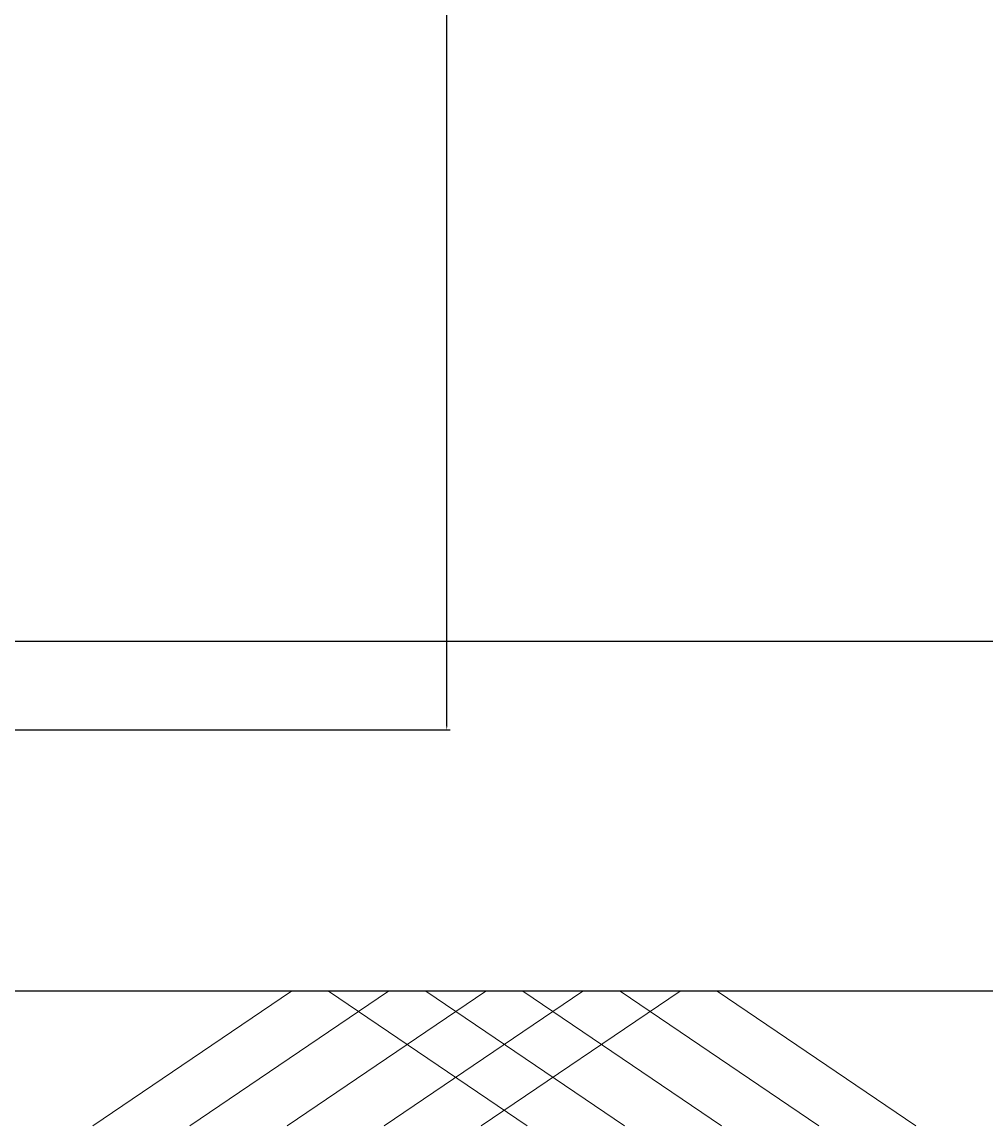
# Model space of a CAD drawing. Units: inches. Extents: x -128 to 854, y -395 to 398.
# Tile 51 of 61: x 368 to 417, y -378 to -322. Entities that reach past the tile are written whole.
import ezdxf

# ---------------------------------------------------------------- set-up
doc = ezdxf.new("R2010")
doc.units = ezdxf.units.IN
doc.header["$MEASUREMENT"] = 0
for name, color, linetype, lineweight in [('A-ANNO-DIMS', 2, 'Continuous', 18), ('C-GRAD', 7, 'Continuous', 25), ('C-GRAD-PATT', 8, 'Continuous', 13)]:
    doc.layers.add(name, color=color, linetype=linetype, lineweight=lineweight)
doc.styles.get("Standard").update_dxf_attribs({"font": 'arial.ttf'})
doc.dimstyles.get("Standard").update_dxf_attribs({"dimtxt": 0.18, "dimasz": 0.18, "dimexe": 0.18, "dimexo": 0.0625, "dimgap": 0.09, "dimtad": 0, "dimtih": 1, "dimtoh": 1, "dimdec": 1, "dimzin": 0, "dimdsep": 46, "dimlunit": 4, "dimtxsty": 'Standard', "dimcen": 0.09, "dimclrd": 1, "dimclre": 2, "dimclrt": 6, "dimadec": 0, "dimazin": 0, "dimtfac": 1, "dimtdec": 1, "dimtofl": 0, "dimtmove": 0, "dimatfit": 3, "dimfxl": 1, "dimtfill": 2, "dimtfillclr": 3, "dimtolj": 1, "dimtzin": 0, "dimarcsym": 0})

# ---------------------------------------------------------------- blocks, each defined once
blk = doc.blocks.new('*D120')
at = {"layer": 'A-ANNO-DIMS', "color": 2, "lineweight": -2, "transparency": 16777216}
for p, q in [((317.902, -178.019), (389.719, -178.019)), ((337.902, -358.019), (389.719, -358.019))]:
    blk.add_line(p, q, dxfattribs=at)
at = {"layer": 'A-ANNO-DIMS', "color": 1, "lineweight": -2, "transparency": 16777216}
for p, q in [((389.539, -178.199), (389.539, -267.837)), ((389.539, -357.839), (389.539, -268.201))]:
    blk.add_line(p, q, dxfattribs=at)
at = {"layer": 'A-ANNO-DIMS', "color": 1, "transparency": 16777216}
for points in [[(389.509, -178.199), (389.569, -178.199), (389.539, -178.019)], [(389.509, -357.839), (389.569, -357.839), (389.539, -358.019)]]:
    blk.add_solid(points, dxfattribs=at)
at = {"layer": 'Defpoints', "color": 0, "transparency": 16777216}
for p in [(317.839, -178.019), (337.839, -358.019), (389.539, -358.019)]:
    blk.add_point(p, dxfattribs=at)
at = {"layer": 'A-ANNO-DIMS', "color": 6, "transparency": 16777216, "insert": (389.539, -268.019), "char_height": 0.18, "attachment_point": 5, "bg_fill": 1, "box_fill_scale": 1.25, "bg_fill_color": 3, "bg_fill_transparency": 0}
blk.add_mtext('\\A1;15\'-0"', dxfattribs=at)
blk = doc.blocks.new('*D134')
at = {"layer": 'A-ANNO-DIMS', "color": 2, "lineweight": -2, "transparency": 16777216}
for p, q in [((418.217, -191.476), (346.3, -191.476)), ((418.217, -371.476), (346.3, -371.476))]:
    blk.add_line(p, q, dxfattribs=at)
at = {"layer": 'A-ANNO-DIMS', "color": 1, "lineweight": -2, "transparency": 16777216}
for p, q in [((346.48, -191.656), (346.48, -281.295)), ((346.48, -371.296), (346.48, -281.658))]:
    blk.add_line(p, q, dxfattribs=at)
at = {"layer": 'A-ANNO-DIMS', "color": 1, "transparency": 16777216}
for points in [[(346.45, -191.656), (346.51, -191.656), (346.48, -191.476)], [(346.45, -371.296), (346.51, -371.296), (346.48, -371.476)]]:
    blk.add_solid(points, dxfattribs=at)
at = {"layer": 'Defpoints', "color": 0, "transparency": 16777216}
for p in [(346.48, -191.476), (418.28, -191.476), (418.28, -371.476)]:
    blk.add_point(p, dxfattribs=at)
at = {"layer": 'A-ANNO-DIMS', "color": 6, "transparency": 16777216, "insert": (346.48, -281.476), "char_height": 0.18, "attachment_point": 5, "bg_fill": 1, "box_fill_scale": 1.25, "bg_fill_color": 3, "bg_fill_transparency": 0}
blk.add_mtext('\\A1;15\'-0"', dxfattribs=at)
blk = doc.blocks.new('*D140')
at = {"layer": 'A-ANNO-DIMS', "color": 2, "lineweight": -2, "transparency": 16777216}
for p, q in [((551.245, -257.476), (346.3, -257.476)), ((551.245, -353.476), (346.3, -353.476))]:
    blk.add_line(p, q, dxfattribs=at)
at = {"layer": 'A-ANNO-DIMS', "color": 1, "lineweight": -2, "transparency": 16777216}
for p, q in [((346.48, -257.656), (346.48, -305.295)), ((346.48, -353.296), (346.48, -305.658))]:
    blk.add_line(p, q, dxfattribs=at)
at = {"layer": 'A-ANNO-DIMS', "color": 1, "transparency": 16777216}
for points in [[(346.45, -257.656), (346.51, -257.656), (346.48, -257.476)], [(346.45, -353.296), (346.51, -353.296), (346.48, -353.476)]]:
    blk.add_solid(points, dxfattribs=at)
at = {"layer": 'Defpoints', "color": 0, "transparency": 16777216}
for p in [(346.48, -257.476), (551.307, -257.476), (551.307, -353.476)]:
    blk.add_point(p, dxfattribs=at)
at = {"layer": 'A-ANNO-DIMS', "color": 6, "transparency": 16777216, "insert": (346.48, -305.476), "char_height": 0.18, "attachment_point": 5, "bg_fill": 1, "box_fill_scale": 1.25, "bg_fill_color": 3, "bg_fill_transparency": 0}
blk.add_mtext('\\A1;8\'-0"', dxfattribs=at)

msp = doc.modelspace()

# ---------------------------------------------------------------- hatches: boundary and pattern name
at = {"layer": 'C-GRAD-PATT'}
h = msp.add_hatch(dxfattribs=at)
h.set_pattern_fill('ANSI31', color=256, scale=22.43157, angle=349.1104, style=0)
h.paths.add_polyline_path([(379.759, -371.476), (404.739, -371.476), (394.513, -378.403), (369.533, -378.403)])
h = msp.add_hatch(dxfattribs=at)
h.set_pattern_fill('ANSI31', color=256, scale=22.43157, angle=100.8896, style=0)
h.paths.add_polyline_path([(379.759, -371.476), (404.739, -371.476), (414.965, -378.403), (389.985, -378.403)])

# ---------------------------------------------------------------- linework, layer by layer
at = {"layer": 'C-GRAD'}
msp.add_line((418.28, -371.476), (370.28, -371.476), dxfattribs=at)

# ---------------------------------------------------------------- dimensions: what is measured, and where the dimension line sits
at = {"layer": 'A-ANNO-DIMS'}
for base, p1, p2, picture, middle in [((389.539, -358.019), (317.839, -178.019), (337.839, -358.019), '*D120', (389.539, -268.019)), ((346.48, -191.476), (418.28, -371.476), (418.28, -191.476), '*D134', (346.48, -281.476)), ((346.48, -257.476), (551.307, -353.476), (551.307, -257.476), '*D140', (346.48, -305.476))]:
    dim = msp.add_linear_dim(base=base, p1=p1, p2=p2, angle=90, dimstyle='Standard', override={"dimdec": 1, "dimlfac": 1, "dimrnd": 0, "dimzin": 1, "dimdsep": 46, "dimlunit": 4, "dimfrac": 2}, dxfattribs=at)
    dim.commit()
    dim.dimension.update_dxf_attribs({"geometry": picture, "text_midpoint": middle})

doc.saveas('drawing.dxf')
